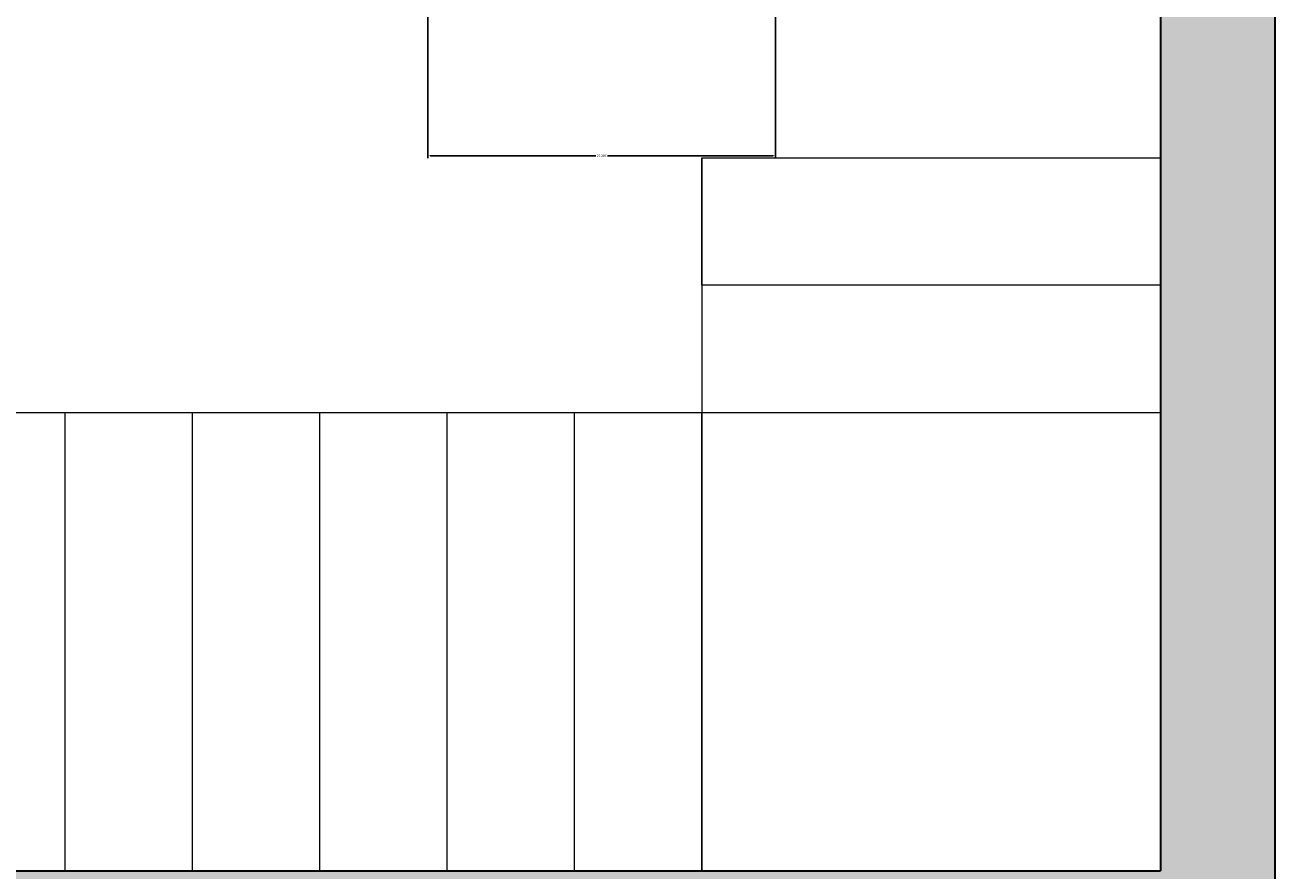
# Model space of a CAD drawing. Units: inches. Extents: x -30 to 437, y -29 to 647.
# Tile 11 of 15: x 308 to 406, y 255 to 321. Entities that reach past the tile are written whole.
import ezdxf

# ---------------------------------------------------------------- set-up
doc = ezdxf.new("R2010")
doc.units = ezdxf.units.IN
doc.header["$MEASUREMENT"] = 0
for name, color, linetype, lineweight in [('A-ANNO-DIMS', 2, 'Continuous', 18), ('A-FLOR-STRS', 7, 'Continuous', 18), ('A-WALL', 7, 'Continuous', 35)]:
    doc.layers.add(name, color=color, linetype=linetype, lineweight=lineweight)
doc.layers.add('A-WALL-PATT', color=251, linetype='Continuous', lineweight=13, true_color=0x636466)
doc.styles.get("Standard").update_dxf_attribs({"font": 'arial.ttf'})
doc.dimstyles.get("Standard").update_dxf_attribs({"dimtxt": 0.18, "dimasz": 0.18, "dimexe": 0.18, "dimexo": 0.0625, "dimgap": 0.09, "dimtad": 0, "dimtih": 1, "dimtoh": 1, "dimdec": 4, "dimzin": 0, "dimdsep": 46, "dimtxsty": 'Standard', "dimcen": 0.09, "dimadec": 0, "dimazin": 0, "dimtfac": 1, "dimtdec": 4, "dimtofl": 0, "dimtmove": 0, "dimatfit": 3, "dimfxl": 1, "dimtolj": 1, "dimtzin": 0, "dimarcsym": 0})

# ---------------------------------------------------------------- blocks, each defined once
blk = doc.blocks.new('*D50')
at = {"layer": 'A-ANNO-DIMS', "color": 0, "lineweight": -2, "transparency": 16777216}
for p, q in [((339.149, 341.543), (339.149, 310.526)), ((366.436, 341.543), (366.436, 310.526)), ((339.329, 310.706), (352.327, 310.706)), ((366.256, 310.706), (353.258, 310.706))]:
    blk.add_line(p, q, dxfattribs=at)
at = {"layer": 'A-ANNO-DIMS', "color": 0, "transparency": 16777216}
for points in [[(339.329, 310.736), (339.329, 310.676), (339.149, 310.706)], [(366.256, 310.736), (366.256, 310.676), (366.436, 310.706)]]:
    blk.add_solid(points, dxfattribs=at)
at = {"layer": 'Defpoints', "color": 0, "transparency": 16777216}
for p in [(339.149, 341.606), (366.436, 341.606), (339.149, 310.706)]:
    blk.add_point(p, dxfattribs=at)
at = {"layer": 'A-ANNO-DIMS', "color": 0, "transparency": 16777216, "insert": (352.792, 310.706), "char_height": 0.18, "attachment_point": 5}
blk.add_mtext('\\A1;27.286', dxfattribs=at)

msp = doc.modelspace()

# ---------------------------------------------------------------- hatches: boundary and pattern name
at = {"layer": 'A-WALL-PATT'}
h = msp.add_hatch(color=256, dxfattribs=at)
h.dxf.hatch_style = 1
h.paths.add_polyline_path([(393.6054, 183.2352), (369.6054, 183.2352), (369.6054, 213.2352), (393.6054, 213.2352), (393.6054, 207.2352), (394.6054, 207.2352), (394.6054, 211.2352), (395.6054, 211.2352), (395.6054, 185.2352), (394.6054, 185.2352), (394.6054, 189.2352), (393.6054, 189.2352)], flags=0)
h.paths.add_polyline_path([(384.6054, 189.2352, -1), (390.6054, 189.2352, -1)], flags=0)
h.paths.add_polyline_path([(385.6054, 189.2352, -1), (389.6054, 189.2352, -1)], flags=0)
h.paths.add_polyline_path([(374.6054, 189.2352, -1), (382.6054, 189.2352, -1)], flags=0)
h.paths.add_polyline_path([(386.6054, 189.2352, -1), (388.6054, 189.2352, -1)], flags=0)
h.paths.add_polyline_path([(375.6054, 189.2352, -1), (381.6054, 189.2352, -1)], flags=0)
h.paths.add_polyline_path([(376.6054, 189.2352, -1), (380.6054, 189.2352, -1)], flags=0)
h.paths.add_polyline_path([(377.6054, 189.2352, -1), (379.6054, 189.2352, -1)], flags=0)
h.paths.add_polyline_path([(390.6054, 195.2352), (374.6054, 195.2352), (374.6054, 201.2352), (390.6054, 201.2352)], flags=0)
h.paths.add_polyline_path([(389.6054, 196.2352), (375.6054, 196.2352), (375.6054, 200.2352), (389.6054, 200.2352)], flags=0)
h.paths.add_polyline_path([(383.6054, 207.2352, -1), (391.6054, 207.2352, -1)], flags=0)
h.paths.add_polyline_path([(384.6054, 207.2352, -1), (390.6054, 207.2352, -1)], flags=0)
h.paths.add_polyline_path([(385.6054, 207.2352, -1), (389.6054, 207.2352, -1)], flags=0)
h.paths.add_polyline_path([(386.6054, 207.2352, -1), (388.6054, 207.2352, -1)], flags=0)
h.paths.add_polyline_path([(375.6054, 207.2352, -1), (381.6054, 207.2352, -1)], flags=0)
h.paths.add_polyline_path([(376.6054, 207.2352, -1), (380.6054, 207.2352, -1)], flags=0)
h.paths.add_polyline_path([(377.6054, 207.2352, -1), (379.6054, 207.2352, -1)], flags=0)
h.paths.add_polyline_path([(305.5437, 160.3663, -0.4142136), (304.0437, 158.8663), (271.0437, 158.8663, -0.4142136), (269.5437, 160.3663), (269.5437, 178.3663, -0.4142136), (271.0437, 179.8663), (304.0437, 179.8663, -0.4142136), (305.5437, 178.3663)], flags=0)
h.paths.add_polyline_path([(304.0437, 165.3663, -0.4142136), (303.0437, 164.3663), (289.2937, 164.3663, -0.4142136), (288.2937, 165.3663), (288.2937, 177.3663, -0.4142136), (289.2937, 178.3663), (303.0437, 178.3663, -0.4142136), (304.0437, 177.3663)], flags=0)
h.paths.add_polyline_path([(296.5437, 171.3663, -1), (295.5437, 171.3663, -1)], flags=0)
h.paths.add_polyline_path([(286.7937, 165.3663, -0.4142136), (285.7937, 164.3663), (272.0437, 164.3663, -0.4142136), (271.0437, 165.3663), (271.0437, 177.3663, -0.4142136), (272.0437, 178.3663), (285.7937, 178.3663, -0.4142136), (286.7937, 177.3663)], flags=0)
h.paths.add_polyline_path([(279.5437, 171.3663, -1), (278.5437, 171.3663, -1)], flags=0)
h.paths.add_polyline_path([(360.6737, 290.5474), (360.6737, 300.5474), (396.6737, 300.5474), (396.6737, 290.5474)], flags=0)
h.paths.add_polyline_path([(259.6737, 124.5474), (259.6737, 114.5474), (171.6737, 114.5474), (171.6737, 124.5474)], flags=0)
h.paths.add_polyline_path([(288.0737, 215.3705), (286.7097, 214.583), (268.7097, 245.7599), (270.0737, 246.5474)], flags=0)
h.paths.add_polyline_path([(259.6737, 168.5474), (256.6737, 168.5474), (256.6737, 173.5474), (256.6737, 179.0224), (255.8753, 177.6395), (224.2956, 195.872, 0.1205374), (220.1737, 179.0224, 0.1205374), (216.0518, 195.872), (184.4721, 177.6395), (183.6737, 179.0224), (215.2836, 197.2724), (216.0821, 195.8895), (216.0518, 195.872, -0.1205374), (220.1737, 179.0224, -0.1205374), (224.2956, 195.872), (224.2653, 195.8895), (225.0638, 197.2724), (256.6737, 179.0224), (256.6737, 173.5474), (259.6737, 173.5474)], flags=0)
h.paths.add_polyline_path([(386.7943, 325.4601), (372.6871, 325.4601), (372.6871, 339.5673), (386.7943, 339.5673)], flags=0)
h.paths.add_polyline_path([(359.5875, 343.7429), (357.7905, 343.7429), (357.7905, 327.9179), (359.3933, 327.9179, 0.4142089), (361.5302, 330.0549), (361.5302, 341.8434, 0.4143616)], flags=0)
h.paths.add_polyline_path([(341.7887, 323.1235, -0.1192167), (340.7839, 323.1235)], flags=0)
h.paths.add_polyline_path([(379.6332, 328.8632), (379.6332, 332.2699), (376.0992, 332.2699, 0.3942773)], flags=0)
h.paths.add_polyline_path([(375.5299, 332.459, -1), (383.8511, 332.459, -1)], flags=0)
h.paths.add_polyline_path([(388.9363, 344.7425), (372.5309, 344.7425, -0.4142136), (370.394, 346.8794), (370.394, 347.5594, -0.3908517), (372.3472, 349.7005, -0.4395101), (370.394, 351.4933), (370.394, 365.1894, -0.4030545), (372.2191, 367.1298, -0.4183945), (370.394, 368.9291), (370.394, 382.6251, -0.4088583), (372.2519, 384.5722, -0.4237732), (370.394, 386.3707), (370.394, 400.0667, -0.3866069), (372.1327, 402.0094), (372.531, 402.0094, -0.4142183), (370.394, 404.1464), (370.394, 404.7778, -0.4142089), (372.5309, 406.9147), (388.9363, 406.9147, -0.4142182), (391.0733, 404.7778), (391.0733, 346.8794, -0.4142136)], flags=0)
edge = h.paths.add_edge_path(flags=0)
edge.add_spline(control_points=[(349.3585, 363.204), (349.0859, 363.204), (348.8133, 363.2227), (348.2712, 363.2973), (348.0016, 363.3531), (347.3533, 363.5328), (346.9776, 363.6755), (346.2445, 364.0308), (345.887, 364.2432), (345.1953, 364.7329), (344.8611, 365.0101), (344.2197, 365.6237), (343.9125, 365.9603), (343.211, 366.8336), (342.8313, 367.3965), (342.1401, 368.6117), (341.8286, 369.2641), (341.2807, 370.64), (341.0443, 371.3636), (340.6522, 372.8619), (340.4964, 373.6367), (340.2695, 375.2158), (340.1983, 376.0203), (340.142, 377.6365), (340.157, 378.4483), (340.2729, 380.0567), (340.3738, 380.8533), (340.6589, 382.4093), (340.8432, 383.1686), (341.2906, 384.629), (341.5538, 385.3301), (342.1531, 386.6544), (342.4891, 387.2776), (343.2266, 388.4288), (343.6281, 388.9567), (344.4879, 389.9012), (344.9463, 390.3178), (345.7981, 390.9428), (346.182, 391.1771), (346.9712, 391.5648), (347.3766, 391.7182), (348.2004, 391.9387), (348.6189, 392.0058), (349.4588, 392.0508), (349.8801, 392.0288), (350.7146, 391.8966), (351.1278, 391.7865), (351.9366, 391.4822), (352.3323, 391.2882), (353.0989, 390.8223), (353.4699, 390.5504), (354.1819, 389.9355), (354.5229, 389.5924), (355.1706, 388.8418), (355.4772, 388.4343), (356.1315, 387.4422), (356.4671, 386.8397), (357.0692, 385.5581), (357.3356, 384.879), (357.7933, 383.4624), (357.9846, 382.725), (358.2875, 381.2112), (358.3992, 380.4349), (358.5404, 378.8643), (358.5699, 378.0699), (358.546, 376.4841), (358.4926, 375.6928), (358.3042, 374.1343), (358.1692, 373.3672), (357.8207, 371.8774), (357.6072, 371.1549), (357.1067, 369.7735), (356.8196, 369.1148), (356.1782, 367.8787), (355.8238, 367.3013), (355.0551, 366.244), (354.6408, 365.7641), (353.7607, 364.9161), (353.2948, 364.5481), (352.445, 364.0149), (352.0701, 363.822), (351.3034, 363.5117), (350.9116, 363.3943), (350.1325, 363.2418), (349.7455, 363.204), (349.3585, 363.204)], knot_values=[3.1415927, 3.1415927, 3.1415927, 3.1415927, 3.2269172, 3.2269172, 3.3122416, 3.3122416, 3.4342667, 3.4342667, 3.5562918, 3.5562918, 3.6783168, 3.6783168, 3.8003419, 3.8003419, 3.9715738, 3.9715738, 4.1428058, 4.1428058, 4.3140377, 4.3140377, 4.4852697, 4.4852697, 4.6565016, 4.6565016, 4.8277335, 4.8277335, 4.9989655, 4.9989655, 5.1701974, 5.1701974, 5.3414293, 5.3414293, 5.5126613, 5.5126613, 5.6838932, 5.6838932, 5.8551252, 5.8551252, 5.9866911, 5.9866911, 6.118257, 6.118257, 6.2498229, 6.2498229, 6.3813888, 6.3813888, 6.5129547, 6.5129547, 6.6445207, 6.6445207, 6.7760866, 6.7760866, 6.9076525, 6.9076525, 7.0392184, 7.0392184, 7.2070156, 7.2070156, 7.3748129, 7.3748129, 7.5426101, 7.5426101, 7.7104073, 7.7104073, 7.8782046, 7.8782046, 8.0460018, 8.0460018, 8.213799, 8.213799, 8.3815962, 8.3815962, 8.5493935, 8.5493935, 8.7171907, 8.7171907, 8.8849879, 8.8849879, 9.0527852, 9.0527852, 9.178207, 9.178207, 9.3036288, 9.3036288, 9.424778, 9.424778, 9.424778, 9.424778], degree=3, periodic=0)
edge.add_line((341.1696, 384.3006), (341.2012, 384.2808))
edge = h.paths.add_edge_path(flags=0)
edge.add_line((344.3353, 388.7801), (344.317, 388.7915))
edge.add_ellipse((349.3585, 377.6204), major_axis=(0, -13.7895), ratio=0.6218602, start_angle=-244.867444, end_angle=-124.769923)
h.paths.add_polyline_path([(163.6737, 163.1474), (132.4968, 145.1474), (131.7093, 146.5114), (162.8862, 164.5114)], flags=0)
h.paths.add_polyline_path([(366.4355, 409.0896, -0.4142367), (364.2985, 406.9525, -0.4913499), (361.5302, 408.8973), (361.5302, 420.6405, 0.4142136), (359.3932, 422.7775), (357.7905, 422.7775), (357.7905, 406.9525), (359.6317, 406.9525, 0.4274103), (361.5332, 408.9757, 0.3986947), (363.6672, 406.9525, 0.519581), (366.4355, 409.0895)], flags=0)
h.paths.add_polyline_path([(386.7943, 410.9671), (372.6871, 410.9671), (372.6871, 425.0742), (386.7943, 425.0742)], flags=0)
h.paths.add_polyline_path([(379.6332, 414.3701), (379.6332, 417.7768), (376.0992, 417.7768, 0.3942773)], flags=0)
h.paths.add_polyline_path([(375.5299, 417.966, -1), (383.8511, 417.966, -1)], flags=0)
h.paths.add_polyline_path([(150.0377, 351.583), (148.6737, 352.3705), (166.6737, 383.5474), (168.0377, 382.7599)], flags=0)
h.paths.add_polyline_path([(91.6737, 234.1974), (66.559, 219.6974), (65.9246, 220.7962), (91.0393, 235.2962)], flags=0)
h.paths.add_polyline_path([(255.4612, 443.5834), (254.6737, 444.9474), (285.8506, 462.9474), (286.6381, 461.5834)], flags=0)
h.paths.add_polyline_path([(176.2737, 394.5474), (158.2737, 425.7243), (159.6377, 426.5118), (177.6377, 395.3349)], flags=0)
h.paths.add_polyline_path([(243.6737, 439.5474), (243.0393, 438.4486), (217.9246, 452.9486), (218.559, 454.0474)], flags=0)
h.paths.add_polyline_path([(38.1264, 269.8429), (40.2408, 269.8429), (40.2408, 270.3508), (38.1264, 270.3508)], flags=0)
h.paths.add_polyline_path([(75.7157, 289.9439), (40.2408, 289.9439), (38.1264, 289.6524), (40.2408, 289.6524)], flags=0)
h.paths.add_polyline_path([(75.7157, 270.0846), (77.6447, 270.0846), (77.6697, 270.1626), (75.7175, 270.1626)], flags=0)
h.paths.add_polyline_path([(80.5373, 293.3002), (33.0467, 293.3002), (13.5054, 293.3002), (13.5054, 351.9244), (29.7898, 351.9244), (80.5373, 351.9244)], flags=0)
h.paths.add_polyline_path([(46.0261, 212.466, -0.5013168), (27.1651, 207.5106), (21.165, 209.5107), (21.165, 206.5107), (22.665, 206.5107), (22.665, 203.5107), (21.165, 203.5107), (21.165, 203.0107), (13.165, 203.0107), (13.165, 224.0107), (21.165, 224.0107), (21.165, 217.5107), (27.1649, 219.5106, -0.5013235), (46.0261, 214.5554, -0.1328909)], flags=0)
h.paths.add_polyline_path([(44.688, 211.8666, -0.4800797), (27.165, 209.5107), (27.165, 217.5107, -0.4800795), (44.688, 215.1547, -0.2150038)], flags=0)
h.paths.add_polyline_path([(19.415, 204.0107), (15.165, 204.0107, -0.4142136), (14.165, 204.7607), (14.165, 222.0107, -0.4142136), (14.915, 223.0107), (19.165, 223.0107, -0.4142136), (20.165, 222.2607), (20.165, 205.0107, -0.4142136)], flags=0)
h.paths.add_polyline_path([(32.7608, 269.0719), (31.8439, 269.0719), (31.8439, 268.6134), (13.5054, 268.6134), (13.5054, 291.5366), (31.8439, 291.5366), (32.7608, 291.0781), (32.7608, 280.9919, -1), (32.7608, 279.1581)], flags=0)
h.paths.add_polyline_path([(40.2408, 360.1436), (38.1264, 360.1436), (38.1264, 359.6357), (40.2408, 359.6357)], flags=0)
h.paths.add_polyline_path([(75.7157, 355.2807), (40.2408, 355.2807), (38.1264, 355.5722), (40.2408, 355.5722), (40.2408, 355.2807), (75.7157, 355.2807), (75.7157, 375.5982), (40.2408, 375.5982), (38.1264, 375.3817), (40.2408, 375.3817), (40.2408, 375.5982), (75.7157, 375.5982), (77.9733, 375.062), (75.7175, 375.062), (75.7175, 374.554)], flags=0)
h.paths.add_polyline_path([(42.8174, 299.814, 0.1386707), (34.1602, 294.603), (14.8081, 294.603), (14.8081, 350.6216), (29.8539, 350.6216, 0.0982206)], flags=0)
h.paths.add_polyline_path([(15.8636, 276.7781, -0.3064017), (20.3757, 283.4499), (20.3483, 290.6726), (31.4014, 290.7146), (31.4309, 282.9124), (26.8287, 282.895, -0.2600628), (30.241, 276.7781, -1)], flags=0)
h.paths.add_polyline_path([(26.1332, 276.7781), (23.0523, 273.6972), (19.9714, 276.7781), (23.0523, 279.8589), (23.0523, 283.9209), (21.3493, 283.9145), (20.7006, 283.5219), (20.6907, 286.1226), (23.2914, 286.1325), (25.8936, 285.7522), (27.1939, 285.7572), (28.4928, 286.1522), (31.0935, 286.1621), (31.0918, 286.6172), (25.6303, 286.5965), (25.616, 290.3675), (31.0775, 290.3882), (31.0918, 286.6172), (31.1034, 283.5614), (28.5027, 283.5515), (25.9005, 283.9317), (23.0523, 283.9209), (23.0523, 279.8589)], flags=0)
h.paths.add_polyline_path([(24.0793, 276.7781, -1), (22.0253, 276.7781, -1)], flags=0)
h.paths.add_polyline_path([(35.7687, 302.2895, -0.4142136), (35.2283, 301.2726), (22.2164, 297.2909, -0.4142136), (21.1995, 297.8313), (15.7317, 315.6996, -0.4142136), (16.2721, 316.7165), (18.8554, 317.507), (15.3721, 328.8904, -0.4142136), (15.9125, 329.9073), (28.9244, 333.889, -0.4142136), (29.9414, 333.3486), (35.4091, 315.4802, -0.4142136), (34.8687, 314.4633), (32.2854, 313.6728)], flags=0)
h.paths.add_polyline_path([(361.3728, 532.6207), (302.7487, 532.6207), (302.7487, 580.1113), (302.7487, 599.6527), (361.3728, 599.6527), (361.3728, 583.3682)], flags=0)
h.paths.add_polyline_path([(370.1, 575.0316), (370.1, 572.9172), (370.6079, 572.9172), (370.6079, 575.0316)], flags=0)
h.paths.add_polyline_path([(385.0466, 537.4423), (385.0466, 572.9172), (384.8302, 575.0316), (384.8302, 572.9172)], flags=0)
h.paths.add_polyline_path([(384.5104, 535.3262), (384.5104, 537.4406), (384.0025, 537.4406), (364.7291, 537.4423), (364.7291, 572.9172), (365.0206, 575.0316), (365.0206, 572.9172), (364.7291, 572.9172), (364.7291, 537.4423), (384.5884, 537.4423), (384.5884, 535.5133)], flags=0)
h.paths.add_polyline_path([(384.5884, 535.5133), (383.4945, 535.164), (383.4945, 537.4406), (382.9866, 535.3262), (382.9866, 537.4406), (383.4945, 535.3262), (383.4945, 537.4406), (384.5884, 537.4406)], flags=0)
h.paths.add_polyline_path([(23.874, 286.8174), (21.0132, 286.8065), (21.0004, 290.1875), (23.8612, 290.1983)], flags=0)
h.paths.add_polyline_path([(242.9824, 511.1667), (234.9824, 511.1667), (234.9824, 517.6667), (228.9825, 515.6667, -0.5013235), (210.1213, 520.622, -0.1328909), (210.1213, 522.7114, -0.5013168), (228.9823, 527.6667), (234.9824, 525.6667), (234.9824, 528.6667), (233.4824, 528.6667), (233.4824, 531.6667), (234.9824, 531.6667), (234.9824, 532.1667), (242.9824, 532.1667)], flags=0)
h.paths.add_polyline_path([(236.9824, 512.1667, -0.4142136), (235.9824, 512.9167), (235.9824, 530.1667, -0.4142136), (236.7324, 531.1667), (240.9824, 531.1667, -0.4142136), (241.9824, 530.4167), (241.9824, 513.1667, -0.4142136), (241.2324, 512.1667)], flags=0)
h.paths.add_polyline_path([(279.533, 537.4423), (279.533, 535.5133), (279.6111, 535.4884), (279.6111, 537.4406)], flags=0)
h.paths.add_polyline_path([(279.2913, 575.0316), (279.2913, 572.9172), (279.7992, 572.9172), (279.7992, 575.0316)], flags=0)
h.paths.add_polyline_path([(211.4594, 520.0227, -0.2150038), (211.4594, 523.3107, -0.4800797), (228.9824, 525.6667), (228.9824, 517.6667, -0.4800795)], flags=0)
h.paths.add_polyline_path([(32.7627, 354.1465), (31.8457, 354.1465), (31.8457, 353.688), (13.5054, 353.688), (13.5054, 376.6134), (31.8457, 376.6134), (32.7627, 376.1549), (32.7627, 366.0677, -1), (32.7627, 364.2337)], flags=0)
h.paths.add_polyline_path([(15.9446, 365.1507, -1), (30.3234, 365.1507, -1)], flags=0)
h.paths.add_polyline_path([(41.213, 428.467), (43.3274, 428.467), (43.3274, 428.9749), (41.213, 428.9749)], flags=0)
h.paths.add_polyline_path([(78.8022, 448.568), (43.3274, 448.568), (41.213, 448.2765), (43.3274, 448.2765)], flags=0)
h.paths.add_polyline_path([(78.8022, 428.7087), (80.7313, 428.7087), (80.7562, 428.7868), (78.804, 428.7868)], flags=0)
h.paths.add_polyline_path([(26.2152, 365.1507), (23.134, 362.0696), (20.0529, 365.1507), (23.134, 368.2319)], flags=0)
h.paths.add_polyline_path([(24.1611, 365.1507, -1), (22.107, 365.1507, -1)], flags=0)
h.paths.add_polyline_path([(309.2625, 570.3406, 0.1386707), (304.0514, 578.9978), (304.0514, 598.3499), (360.07, 598.3499), (360.07, 583.3041, 0.0982206)], flags=0)
h.paths.add_polyline_path([(246.6737, 552.5474), (129.6737, 552.5474), (129.6737, 606.5474), (246.6737, 606.5474)], flags=16)
h.paths.add_polyline_path([(373.6822, 580.3953), (363.595, 580.3953), (363.595, 581.3123), (363.1365, 581.3123), (363.1365, 599.6527), (386.0619, 599.6527), (386.0619, 581.3123), (385.6034, 580.3953), (375.5162, 580.3953, -1)], flags=0)
h.paths.add_polyline_path([(83.6239, 451.9244), (36.1333, 451.9244), (16.5919, 451.9244), (16.5919, 510.5485), (32.8764, 510.5485), (83.6239, 510.5485)], flags=0)
h.paths.add_polyline_path([(367.4098, 590.024, -1), (381.7886, 590.024, -1)], flags=0)
h.paths.add_polyline_path([(374.5992, 586.9428), (371.518, 590.024), (374.5992, 593.1052), (377.6803, 590.024)], flags=0)
h.paths.add_polyline_path([(373.5721, 590.024, -1), (375.6262, 590.024, -1)], flags=0)
h.paths.add_polyline_path([(324.9287, 577.7489, -0.4142136), (323.9118, 578.2893), (323.1212, 580.8726), (311.7379, 577.3893, -0.4142136), (310.721, 577.9297), (306.7393, 590.9416, -0.4142136), (307.2797, 591.9585), (325.1481, 597.4263, -0.4142136), (326.165, 596.8859), (326.9555, 594.3026), (338.3388, 597.7859, -0.4142136), (339.3557, 597.2455), (343.3374, 584.2336, -0.4142136), (342.797, 583.2167)], flags=0)
h.paths.add_polyline_path([(300.5265, 580.3972), (290.4404, 580.3972, -1), (288.6065, 580.3972), (278.5203, 580.3972), (278.5203, 581.3142), (278.0619, 581.3142), (278.0619, 599.6527), (300.985, 599.6527), (300.985, 581.3142)], flags=0)
h.paths.add_polyline_path([(300.163, 581.7567), (292.3609, 581.7271), (292.3434, 586.3294, -0.7556792), (279.0378, 590.1057, -0.8253673), (292.8983, 592.7823), (300.1211, 592.8097)], flags=0)
h.paths.add_polyline_path([(299.8367, 582.0805), (296.0656, 582.0662), (293.0098, 582.0546), (292.9999, 584.6553), (293.3802, 587.2575), (293.3694, 590.1057), (289.3074, 590.1057), (286.2265, 587.0248), (283.1456, 590.1057), (286.2265, 593.1866), (289.3074, 590.1057), (293.3694, 590.1057), (293.3629, 591.8088), (292.9703, 592.4575), (295.5711, 592.4673), (295.5809, 589.8666), (295.2007, 587.2644), (295.2056, 585.9641), (295.6006, 584.6652), (295.6105, 582.0645), (296.0656, 582.0662), (296.0449, 587.5277), (299.8159, 587.542)], flags=0)
h.paths.add_polyline_path([(285.1995, 590.1057, -1), (287.2535, 590.1057, -1)], flags=0)
h.paths.add_polyline_path([(299.6467, 589.2969), (296.2658, 589.284), (296.255, 592.1448), (299.6359, 592.1576)], flags=0)
h.paths.add_polyline_path([(35.8473, 427.696), (34.9304, 427.696), (34.9304, 427.2376), (16.5919, 427.2376), (16.5919, 450.1607), (34.9304, 450.1607), (35.8473, 449.7022), (35.8473, 439.6161, -1), (35.8473, 437.7822)], flags=0)
h.paths.add_polyline_path([(18.9502, 435.4022, -0.3064017), (23.4623, 442.074), (23.4349, 449.2968), (34.4879, 449.3387), (34.5175, 441.5366), (29.9152, 441.5191, -0.2600628), (33.3275, 435.4022, -1)], flags=0)
h.paths.add_polyline_path([(29.2197, 435.4022), (26.1389, 432.3213), (23.058, 435.4022), (26.1389, 438.4831), (26.1389, 442.5451), (24.4358, 442.5386), (23.7871, 442.1461), (23.7772, 444.7468), (26.378, 444.7566), (28.9801, 444.3764), (30.2805, 444.3813), (31.5794, 444.7764), (34.1801, 444.7862), (34.1784, 445.2413), (28.7169, 445.2206), (28.7026, 448.9917), (34.164, 449.0124), (34.1784, 445.2413), (34.1899, 442.1855), (31.5892, 442.1756), (28.987, 442.5559), (26.1389, 442.5451), (26.1389, 438.4831)], flags=0)
h.paths.add_polyline_path([(27.1658, 435.4022, -1), (25.1119, 435.4022, -1)], flags=0)
h.paths.add_polyline_path([(45.904, 458.4382, 0.1386707), (37.2467, 453.2271), (17.8947, 453.2271), (17.8947, 509.2457), (32.9405, 509.2457, 0.0982206)], flags=0)
h.paths.add_polyline_path([(26.9605, 445.4415), (24.0997, 445.4307), (24.0869, 448.8116), (26.9477, 448.8225)], flags=0)
h.paths.add_polyline_path([(38.3149, 459.8967), (25.3029, 455.915, -0.4142136), (24.286, 456.4554), (18.8183, 474.3238, -0.4142136), (19.3586, 475.3407), (21.942, 476.1312), (18.4587, 487.5145, -0.4142136), (18.999, 488.5314), (32.011, 492.5131, -0.4142136), (33.0279, 491.9727), (38.4957, 474.1044, -0.4142136), (37.9553, 473.0875), (35.3719, 472.297), (38.8553, 460.9136, -0.4142136)], flags=0)
h.paths.add_polyline_path([(43.3274, 518.7678), (41.213, 518.7678), (41.213, 518.2598), (43.3274, 518.2598)], flags=0)
h.paths.add_polyline_path([(78.8022, 513.9049), (43.3274, 513.9049), (41.213, 514.1964), (43.3274, 514.1964), (43.3274, 513.9049), (78.8022, 513.9049), (78.8022, 534.2223), (43.3274, 534.2223), (41.213, 534.0059), (43.3274, 534.0059), (43.3274, 534.2223), (78.8022, 534.2223), (81.0599, 533.6861), (78.804, 533.6861), (78.804, 533.1782)], flags=0)
h.paths.add_polyline_path([(121.6737, 556.8974), (121.0393, 555.7986), (95.9246, 570.2986), (96.559, 571.3974)], flags=0)
h.paths.add_polyline_path([(35.8493, 512.7707), (34.9322, 512.7707), (34.9322, 512.3122), (16.5919, 512.3122), (16.5919, 535.2376), (34.9322, 535.2376), (35.8493, 534.7791), (35.8493, 524.6919, -1), (35.8493, 522.8579)], flags=0)
h.paths.add_polyline_path([(19.0312, 523.7749, -1), (33.41, 523.7749, -1)], flags=0)
h.paths.add_polyline_path([(26.2206, 520.6937), (23.1394, 523.7749), (26.2206, 526.8561), (29.3018, 523.7749)], flags=0)
h.paths.add_polyline_path([(25.1935, 523.7749, -1), (27.2476, 523.7749, -1)], flags=0)
h.paths.add_polyline_path([(28.4381, 586.0173), (22.438, 588.0173), (22.438, 585.0173), (23.938, 585.0173), (23.938, 582.0173), (22.438, 582.0173), (22.438, 581.5173), (14.438, 581.5173), (14.438, 602.5173), (22.438, 602.5173), (22.438, 596.0173), (28.4379, 598.0173, -0.5013235), (47.2992, 593.062, -0.1328909), (47.2992, 590.9726, -0.5013168)], flags=0)
h.paths.add_polyline_path([(28.438, 588.0174), (28.438, 596.0173, -0.4800795), (45.961, 593.6614, -0.2150038), (45.961, 590.3733, -0.4800797)], flags=0)
h.paths.add_polyline_path([(20.688, 582.5173), (16.438, 582.5173, -0.4142136), (15.438, 583.2673), (15.438, 600.5173, -0.4142136), (16.188, 601.5173), (20.438, 601.5173, -0.4142136), (21.438, 600.7673), (21.438, 583.5173, -0.4142136)], flags=0)
h.paths.add_polyline_path([(171.6737, 2.0474), (171.6737, 104.5474), (259.6737, 104.5474), (259.6737, 148.5474), (396.6737, 148.5474), (396.6737, 2.0474), (405.6737, 2.0474), (405.6737, 615.5474), (1.6737, 615.5474), (1.6737, 2.0474)])
h.paths.add_polyline_path([(171.6737, 104.5474), (259.6737, 104.5474), (259.6737, 210.5474), (264.6737, 210.5474), (264.6737, 153.5474), (396.6737, 153.5474), (396.6737, 249.5474), (264.6737, 249.5474), (264.6737, 246.5474), (259.6737, 246.5474), (259.6737, 254.5474), (396.6737, 254.5474), (396.6737, 434.5474), (290.6737, 434.5474), (290.6737, 439.5474), (396.6737, 439.5474), (396.6737, 606.5474), (251.6737, 606.5474), (251.6737, 439.5474), (254.6737, 439.5474), (254.6737, 434.5474), (243.6737, 434.5474), (243.6737, 439.5474), (246.6737, 439.5474), (246.6737, 547.5474), (186.6737, 547.5474), (186.6737, 439.5474), (214.6737, 439.5474), (214.6737, 434.5474), (186.6737, 434.5474), (186.6737, 430.5474), (181.6737, 430.5474), (181.6737, 547.5474), (121.6737, 547.5474), (121.6737, 552.5474), (124.6737, 552.5474), (124.6737, 606.5474), (10.6737, 606.5474), (10.6737, 552.5474), (92.6737, 552.5474), (92.6737, 547.5474), (10.6737, 547.5474), (10.6737, 391.5474), (181.6737, 391.5474), (181.6737, 394.5474), (186.6737, 394.5474), (186.6737, 386.5474), (171.6737, 386.5474), (171.6737, 383.5474), (166.6737, 383.5474), (166.6737, 386.5474), (10.6737, 386.5474), (10.6737, 238.5474), (62.6737, 238.5474), (62.6737, 233.5474), (10.6737, 233.5474), (10.6737, 173.5474), (94.6737, 173.5474), (94.6737, 233.5474), (91.6737, 233.5474), (91.6737, 238.5474), (166.6737, 238.5474), (166.6737, 347.5474), (171.6737, 347.5474), (171.6737, 233.5474), (99.6737, 233.5474), (99.6737, 173.5474), (127.6737, 173.5474), (127.6737, 168.5474), (10.6737, 168.5474), (10.6737, 11.0474), (166.6737, 11.0474), (166.6737, 168.5474), (163.6737, 168.5474), (163.6737, 173.5474), (183.6737, 173.5474), (183.6737, 168.5474), (171.6737, 168.5474)])

# ---------------------------------------------------------------- linework, layer by layer
at = {"layer": 'A-FLOR-STRS'}
for p, q in [((360.6737, 310.5474), (360.6737, 254.5474)), ((360.6737, 300.5474), (360.6737, 310.5474)), ((360.6737, 310.5474), (396.6737, 310.5474)), ((396.6737, 300.5474), (360.6737, 300.5474)), ((396.6737, 290.5474), (396.6737, 300.5474)), ((270.6737, 290.5474), (396.6737, 290.5474)), ((310.6737, 254.5474), (310.6737, 290.5474)), ((320.6737, 254.5474), (320.6737, 290.5474)), ((330.6737, 254.5474), (330.6737, 290.5474)), ((340.6737, 254.5474), (340.6737, 290.5474)), ((350.6737, 254.5474), (350.6737, 290.5474)), ((360.6737, 254.5474), (360.6737, 290.5474))]:
    msp.add_line(p, q, dxfattribs=at)
at = {"layer": 'A-WALL'}
for p in [(396.6737, 434.5474), (259.6737, 254.5474)]:
    msp.add_line(p, (396.6737, 254.5474), dxfattribs=at)
msp.add_lwpolyline([(171.6737, 2.0474), (1.6737, 2.0474), (1.6737, 615.5474), (405.6737, 615.5474), (405.6737, 2.0474), (396.6737, 2.0474)], dxfattribs=at)

# ---------------------------------------------------------------- dimensions: what is measured, and where the dimension line sits
at = {"layer": 'A-ANNO-DIMS'}
dim = msp.add_linear_dim(base=(339.1493, 310.706), p1=(366.4355, 341.606), p2=(339.1493, 341.606), angle=180, dimstyle='Standard', override={"dimdec": 3, "dimlfac": 1, "dimrnd": 0, "dimzin": 0, "dimdsep": 46, "dimlunit": 2}, dxfattribs=at)
dim.commit()
dim.dimension.update_dxf_attribs({"geometry": '*D50', "text_midpoint": (352.7924, 310.706)})

doc.saveas('drawing.dxf')
